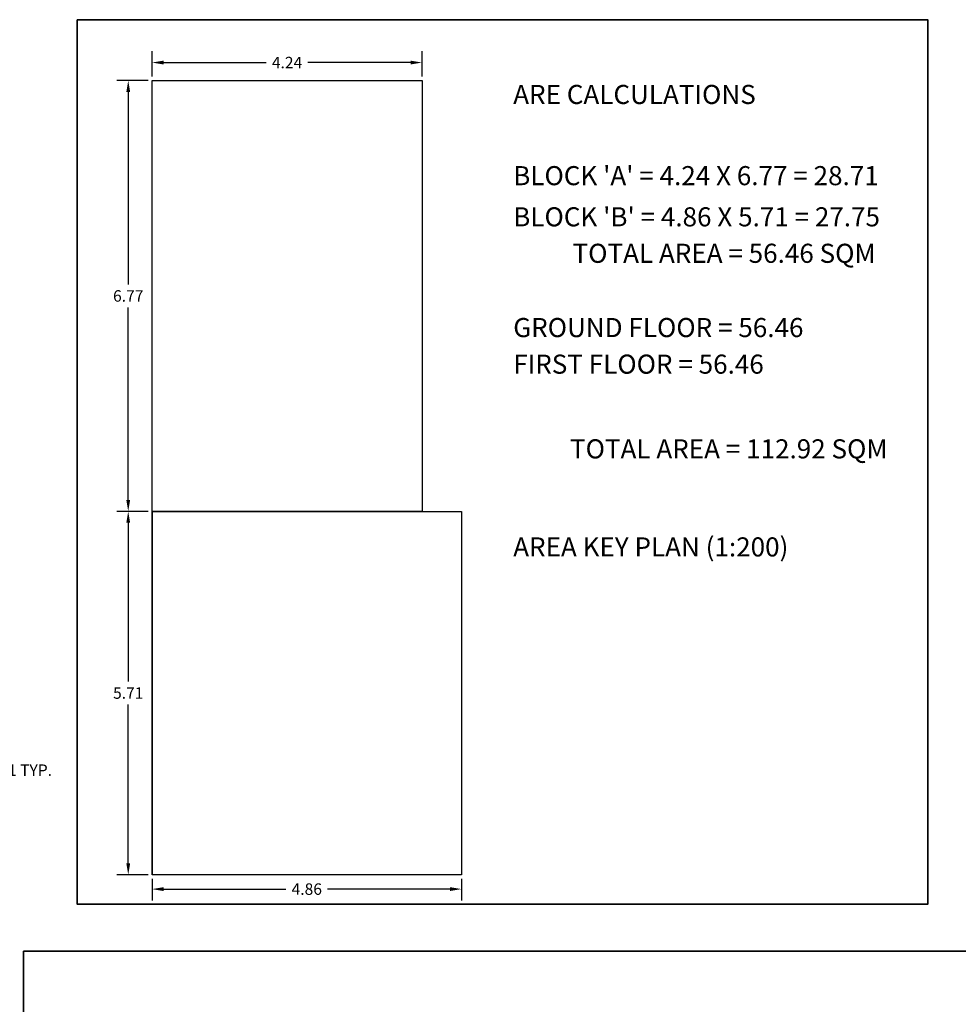
# Model space of a CAD drawing. Units: metres. Extents: x 8.1 to 56.2, y -9.3 to 36.3.
# Tile 4 of 6: x 22.5 to 37.2, y 9.1 to 24.5. Entities that reach past the tile are written whole.
import ezdxf

# ---------------------------------------------------------------- set-up
doc = ezdxf.new("R2010")
doc.units = ezdxf.units.M
doc.header["$LTSCALE"] = 0.01
doc.header["$MEASUREMENT"] = 0
for name, color, linetype, lineweight in [('A-ANNO-DIMS', 2, 'Continuous', 18), ('A-ANNO-TEXT', 7, 'Continuous', 18), ('A-ANNO-TTLB', 7, 'Continuous', 35), ('A-AREA', 6, 'Continuous', 25)]:
    doc.layers.add(name, color=color, linetype=linetype, lineweight=lineweight)
doc.styles.get("Standard").update_dxf_attribs({"font": 'arial.ttf'})
doc.dimstyles.get("Standard").update_dxf_attribs({"dimtxt": 0.18, "dimasz": 0.18, "dimexe": 0.18, "dimexo": 0.0625, "dimgap": 0.09, "dimtad": 0, "dimtih": 1, "dimtoh": 1, "dimzin": 0, "dimdsep": 46, "dimtxsty": 'Standard', "dimcen": 0.09, "dimadec": 0, "dimazin": 0, "dimtfac": 1, "dimtofl": 0, "dimtmove": 0, "dimatfit": 3, "dimfxl": 1, "dimtolj": 1, "dimtzin": 0, "dimarcsym": 0})

# ---------------------------------------------------------------- blocks, each defined once
blk = doc.blocks.new('*D7')
at = {"layer": 'A-ANNO-DIMS', "color": 0, "lineweight": -2, "transparency": 16777216}
for p, q in [((24.587, 23.635), (24.587, 24.035)), ((28.827, 23.635), (28.827, 24.035)), ((24.767, 23.855), (26.38, 23.855)), ((28.647, 23.855), (27.034, 23.855))]:
    blk.add_line(p, q, dxfattribs=at)
at = {"layer": 'A-ANNO-DIMS', "color": 0, "transparency": 16777216}
for points in [[(24.767, 23.885), (24.767, 23.825), (24.587, 23.855)], [(28.647, 23.885), (28.647, 23.825), (28.827, 23.855)]]:
    blk.add_solid(points, dxfattribs=at)
at = {"layer": 'Defpoints', "color": 0, "transparency": 16777216}
for p in [(28.827, 23.855), (24.587, 23.573), (28.827, 23.573)]:
    blk.add_point(p, dxfattribs=at)
at = {"layer": 'A-ANNO-DIMS', "color": 0, "transparency": 16777216, "insert": (26.707, 23.855), "char_height": 0.18, "attachment_point": 5}
blk.add_mtext('\\A1;4.24', dxfattribs=at)
blk = doc.blocks.new('*D8')
at = {"layer": 'A-ANNO-DIMS', "color": 0, "lineweight": -2, "transparency": 16777216}
for p, q in [((24.525, 23.573), (24.033, 23.573)), ((24.213, 23.393), (24.213, 20.369)), ((24.213, 16.983), (24.213, 20.006)), ((24.525, 16.803), (24.033, 16.803))]:
    blk.add_line(p, q, dxfattribs=at)
at = {"layer": 'A-ANNO-DIMS', "color": 0, "transparency": 16777216}
for points in [[(24.183, 23.393), (24.243, 23.393), (24.213, 23.573)], [(24.183, 16.983), (24.243, 16.983), (24.213, 16.803)]]:
    blk.add_solid(points, dxfattribs=at)
at = {"layer": 'Defpoints', "color": 0, "transparency": 16777216}
for p in [(24.587, 23.573), (24.213, 16.803), (24.587, 16.803)]:
    blk.add_point(p, dxfattribs=at)
at = {"layer": 'A-ANNO-DIMS', "color": 0, "transparency": 16777216, "insert": (24.213, 20.188), "char_height": 0.18, "attachment_point": 5}
blk.add_mtext('\\A1;6.77', dxfattribs=at)
blk = doc.blocks.new('*D9')
at = {"layer": 'A-ANNO-DIMS', "color": 0, "lineweight": -2, "transparency": 16777216}
for p, q in [((24.525, 16.803), (24.033, 16.803)), ((24.213, 16.623), (24.213, 14.129)), ((24.213, 11.273), (24.213, 13.766)), ((24.525, 11.093), (24.033, 11.093))]:
    blk.add_line(p, q, dxfattribs=at)
at = {"layer": 'A-ANNO-DIMS', "color": 0, "transparency": 16777216}
for points in [[(24.183, 16.623), (24.243, 16.623), (24.213, 16.803)], [(24.183, 11.273), (24.243, 11.273), (24.213, 11.093)]]:
    blk.add_solid(points, dxfattribs=at)
at = {"layer": 'Defpoints', "color": 0, "transparency": 16777216}
for p in [(24.213, 16.803), (24.587, 16.803), (24.587, 11.093)]:
    blk.add_point(p, dxfattribs=at)
at = {"layer": 'A-ANNO-DIMS', "color": 0, "transparency": 16777216, "insert": (24.213, 13.948), "char_height": 0.18, "attachment_point": 5}
blk.add_mtext('\\A1;5.71', dxfattribs=at)
blk = doc.blocks.new('*D10')
at = {"layer": 'A-ANNO-DIMS', "color": 0, "lineweight": -2, "transparency": 16777216}
for p, q in [((24.587, 11.03), (24.587, 10.687)), ((29.447, 11.03), (29.447, 10.687)), ((24.767, 10.867), (26.69, 10.867)), ((29.267, 10.867), (27.344, 10.867))]:
    blk.add_line(p, q, dxfattribs=at)
at = {"layer": 'A-ANNO-DIMS', "color": 0, "transparency": 16777216}
for points in [[(24.767, 10.897), (24.767, 10.837), (24.587, 10.867)], [(29.267, 10.897), (29.267, 10.837), (29.447, 10.867)]]:
    blk.add_solid(points, dxfattribs=at)
at = {"layer": 'Defpoints', "color": 0, "transparency": 16777216}
for p in [(24.587, 11.093), (29.447, 11.093), (29.447, 10.867)]:
    blk.add_point(p, dxfattribs=at)
at = {"layer": 'A-ANNO-DIMS', "color": 0, "transparency": 16777216, "insert": (27.017, 10.867), "char_height": 0.18, "attachment_point": 5}
blk.add_mtext('\\A1;4.86', dxfattribs=at)
blk = doc.blocks.new('*D47')
at = {"layer": 'A-ANNO-DIMS', "color": 0, "lineweight": -2, "ltscale": 0.01, "transparency": 16777216}
for p, q in [((20.553, 12.556), (20.553, 12.736)), ((20.553, 12.736), (20.733, 12.736)), ((20.611, 12.556), (20.373, 12.556)), ((20.553, 11.928), (20.553, 12.376)), ((20.611, 11.748), (20.373, 11.748))]:
    blk.add_line(p, q, dxfattribs=at)
at = {"layer": 'A-ANNO-DIMS', "color": 0, "ltscale": 0.01, "transparency": 16777216}
for points in [[(20.523, 12.376), (20.583, 12.376), (20.553, 12.556)], [(20.523, 11.928), (20.583, 11.928), (20.553, 11.748)]]:
    blk.add_solid(points, dxfattribs=at)
at = {"layer": 'Defpoints', "color": 0, "ltscale": 0.01, "transparency": 16777216}
for p in [(20.553, 12.556), (20.674, 12.556), (20.674, 11.748)]:
    blk.add_point(p, dxfattribs=at)
at = {"layer": 'A-ANNO-DIMS', "color": 0, "ltscale": 0.01, "transparency": 16777216, "insert": (21.956, 12.736), "char_height": 0.18, "attachment_point": 5}
blk.add_mtext('\\A1;WINDOW 0.81 TYP.', dxfattribs=at)

msp = doc.modelspace()

# ---------------------------------------------------------------- linework, layer by layer
at = {"layer": 'A-ANNO-TTLB'}
for points in [[(23.411, 24.529), (36.768, 24.529), (36.768, 10.629), (23.411, 10.629)], [(22.566, 9.894), (52.195, 9.894), (52.195, -9.317), (22.566, -9.317)]]:
    msp.add_lwpolyline(points, close=True, dxfattribs=at)
at = {"layer": 'A-AREA'}
msp.add_line((24.587, 16.803), (24.587, 11.093), dxfattribs=at)
for points in [[(24.587, 23.573), (28.827, 23.573), (28.827, 16.803), (24.587, 16.803)], [(24.587, 16.803), (29.447, 16.803), (29.447, 11.093), (24.587, 11.093)]]:
    msp.add_lwpolyline(points, close=True, dxfattribs=at)

# ---------------------------------------------------------------- texts
at = {"layer": 'A-ANNO-TEXT', "char_height": 0.3, "attachment_point": 1}
for s, width, insert in [('ARE CALCULATIONS', 5.13719, (30.259, 23.504)), ("BLOCK 'A' = 4.24 X 6.77 = 28.71", 6.38323, (30.259, 22.228)), ("BLOCK 'B' = 4.86 X 5.71 = 27.75", 7.53894, (30.259, 21.581)), ('TOTAL AREA = 56.46 SQM', 6.39447, (31.191, 21.008)), ('GROUND FLOOR = 56.46', 5.23743, (30.259, 19.841)), ('FIRST FLOOR = 56.46', 4.63851, (30.259, 19.266)), ('TOTAL AREA = 112.92 SQM', 5.62593, (31.151, 17.935)), ('{\\fArial|b1|i0|c0|p34;AREA KEY PLAN (1:200)}', 5.26946, (30.259, 16.394))]:
    msp.add_mtext_dynamic_manual_height_columns(s, width=width, gutter_width=1, heights=[0], dxfattribs=dict(at, insert=insert))

# ---------------------------------------------------------------- dimensions: what is measured, and where the dimension line sits
at = {"layer": 'A-ANNO-DIMS'}
for base, p1, p2, picture, middle in [((28.827, 23.855), (24.587, 23.573), (28.827, 23.573), '*D7', (26.707, 23.855)), ((29.447, 10.867), (24.587, 11.093), (29.447, 11.093), '*D10', (27.017, 10.867))]:
    dim = msp.add_linear_dim(base=base, p1=p1, p2=p2, dimstyle='Standard', override={"dimclrd": 0, "dimclre": 0, "dimclrt": 0}, dxfattribs=at)
    dim.commit()
    dim.dimension.update_dxf_attribs({"geometry": picture, "text_midpoint": middle})
for p1, picture, middle in [((24.587, 23.573), '*D8', (24.213, 20.188)), ((24.587, 11.093), '*D9', (24.213, 13.948))]:
    dim = msp.add_linear_dim(base=(24.213, 16.803), p1=p1, p2=(24.587, 16.803), angle=90, dimstyle='Standard', override={"dimclrd": 0, "dimclre": 0, "dimclrt": 0}, dxfattribs=at)
    dim.commit()
    dim.dimension.update_dxf_attribs({"geometry": picture, "text_midpoint": middle})
at = {"layer": 'A-ANNO-DIMS', "ltscale": 0.01}
dim = msp.add_linear_dim(base=(20.553, 12.556), p1=(20.674, 11.748), p2=(20.674, 12.556), angle=90, text='WINDOW <> TYP.', dimstyle='Standard', override={"dimdec": 2, "dimrnd": 0, "dimzin": 0, "dimlunit": 2}, dxfattribs=at)
dim.commit()
dim.dimension.update_dxf_attribs({"geometry": '*D47', "text_midpoint": (21.956, 12.736)})

doc.saveas('drawing.dxf')
